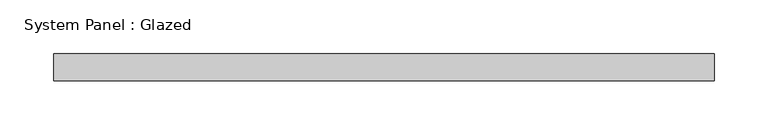
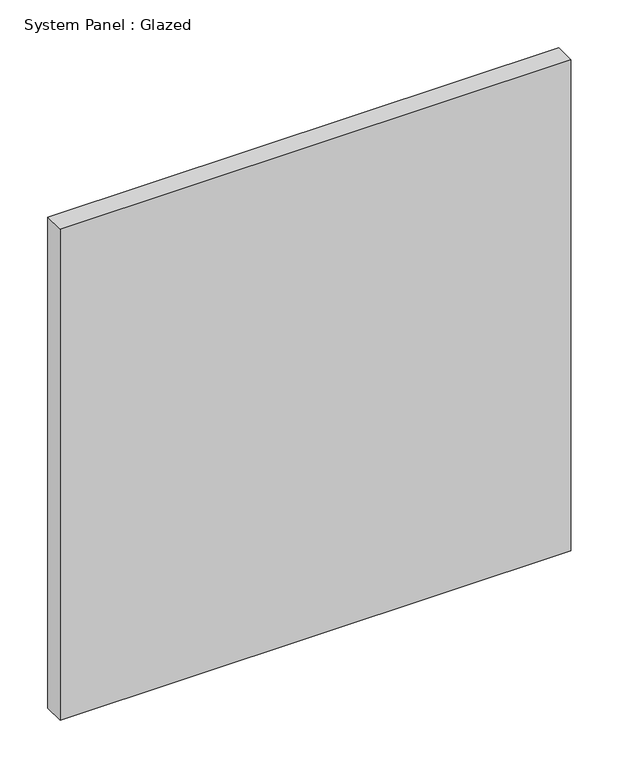
"""IFC4 building model written with IfcOpenShell, lengths in millimetres: plate geometry, System Panel : Glazed."""

from ifc_helpers import new_model, si_unit, origin, origin_with_axes, place, context, project, spatial, polyline, outline, extrude, source, transform, mapped, element, save


def system_panel_glazed_b9962699(model_context):
    return source(origin(), model_context, "Body", "SweptSolid", [
        extrude(outline(polyline([(307.975, 19.05), (-307.975, 19.05), (-307.975, 44.45), (307.975, 44.45), (307.975, 19.05)])), origin_with_axes(), (0.0, 0.0, 1.0), 625.9402035),
    ])


if __name__ == "__main__":
    model = new_model("IFC4")
    model_context = context("Model", 3, world=origin())
    ifc_project = project(units=[si_unit("LENGTHUNIT", "METRE", prefix="MILLI")], contexts=[model_context])
    site = spatial("IfcSite", under=ifc_project)
    building = spatial("IfcBuilding", under=site)
    placement = place(None, origin())
    system_panel_glazed_shape = system_panel_glazed_b9962699(model_context)
    element("IfcPlate", 1, ObjectType="System Panel : Glazed", at=placement, inside=building, context=model_context, shape_type="MappedRepresentation", body=[
        mapped(system_panel_glazed_shape, transform((0.0, 0.0, 0.0), x_axis=(1.0, 0.0, 0.0), y_axis=(0.0, 1.0, 0.0), z_axis=(0.0, 0.0, 1.0))),
    ])
    save(model, "model.ifc")

# Revit data of these elements
# Type "System Panel : Glazed"
#   Construction Type Id = "GSP4R"
#   Analytic Construction = "1/8 in Pilkington single glazing"
#   Visual Light Transmittance = 0.9
#   Solar Heat Gain Coefficient = 0.86
#   Heat Transfer Coefficient (U) = 1.18115 BTU/(h·ft²·°F)
#   Define Thermal Properties by = 1
# Element 1 (IfcPlate, "System Panel : Glazed")
#   Materials on its faces: "Glass"
# Materials
#   "Glass": class "Glass", colour RGB 0 128 192, transparency 0.75, Description = "Soda Lime Glass", Cost = 0
